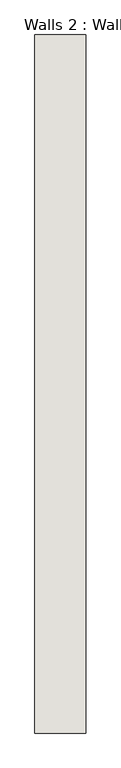
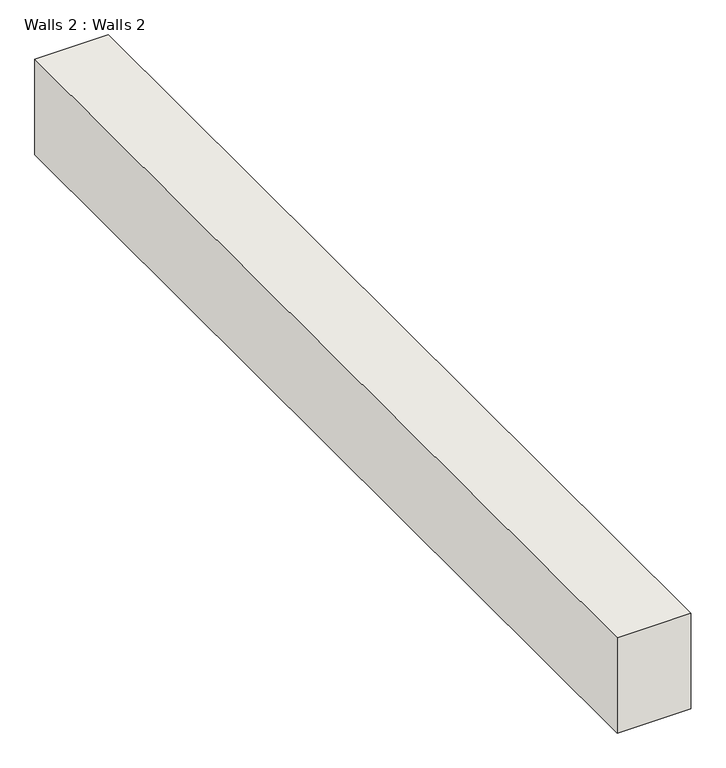
"""IFC4 building model written with IfcOpenShell, lengths in millimetres: wall geometry, Walls 2 : Walls 2."""

from ifc_helpers import new_model, si_unit, frame, origin, place, context, project, spatial, polyline, outline, extrude, source, transform, mapped, element, save


def walls_2_walls_2_fbce2fc9(model_context):
    return source(origin(), model_context, "Body", "SweptSolid", [
        extrude(outline(polyline([(-6234.5683714, 5567.8900371), (-6234.5683714, -528.1099629), (-6678.3379015, -528.1099629), (-6678.3379015, 5567.8900371), (-6234.5683714, 5567.8900371)])), frame((0.0, 0.0, 8991.6), z_axis=(0.0, 0.0, 1.0), x_axis=(1.0, 0.0, 0.0)), (0.0, 0.0, 1.0), 609.6),
    ])


if __name__ == "__main__":
    model = new_model("IFC4")
    model_context = context("Model", 3, world=origin())
    ifc_project = project(units=[si_unit("LENGTHUNIT", "METRE", prefix="MILLI")], contexts=[model_context])
    site = spatial("IfcSite", under=ifc_project)
    building = spatial("IfcBuilding", under=site)
    placement = place(None, origin())
    walls_2_walls_2_shape = walls_2_walls_2_fbce2fc9(model_context)
    element("IfcWall", 1, ObjectType="Walls 2 : Walls 2", at=placement, inside=building, context=model_context, shape_type="MappedRepresentation", body=[
        mapped(walls_2_walls_2_shape, transform((0.0, 0.0, 0.0), x_axis=(1.0, 0.0, 0.0), y_axis=(0.0, 1.0, 0.0), z_axis=(0.0, 0.0, 1.0))),
    ])
    save(model, "model.ifc")

# Revit data of these elements
# Element 1 (IfcWall, "Walls 2 : Walls 2")
#   Materials on its faces: "Default Wall"
# Materials
#   "Default Wall": colour RGB 128 128 128, transparency 0
